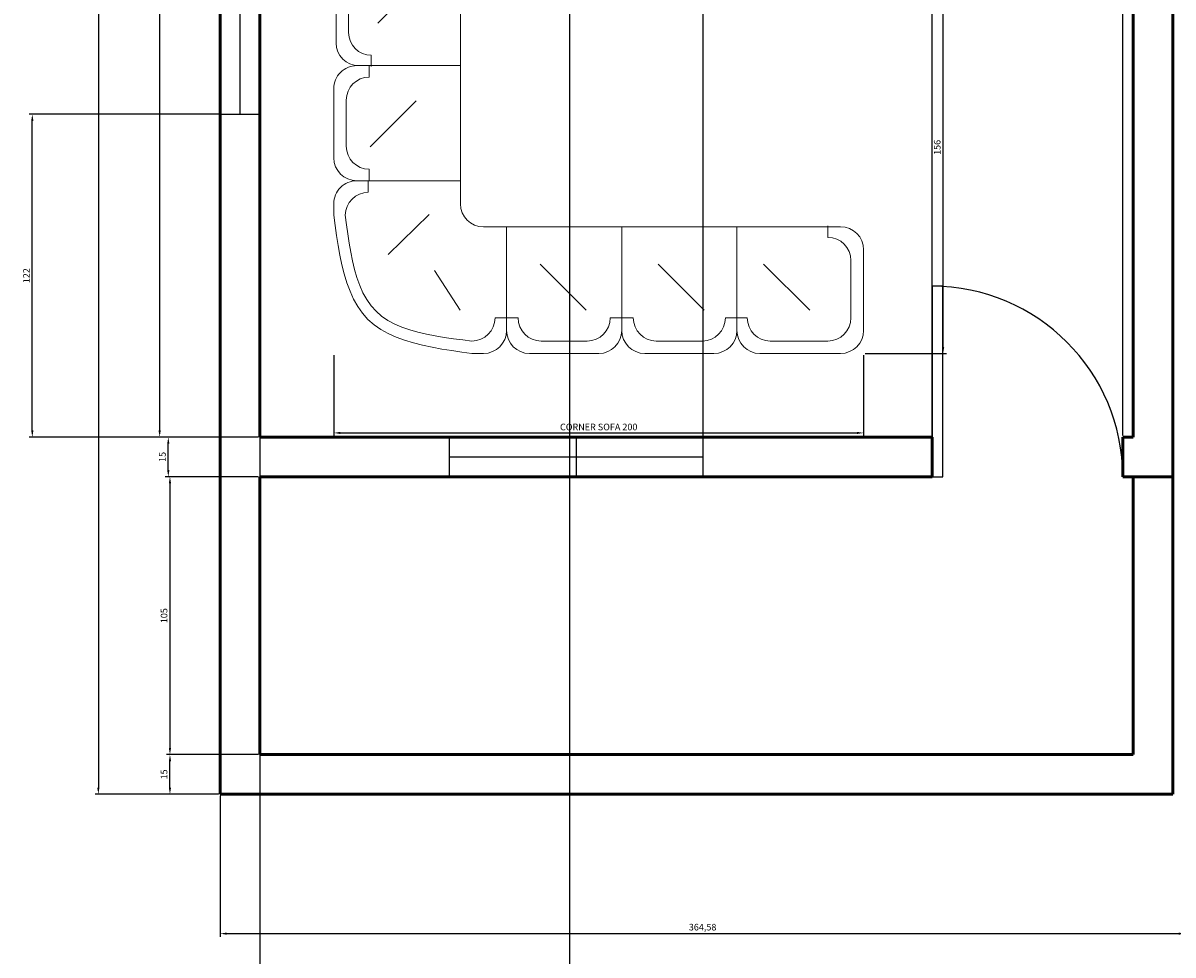
# Model space of a CAD drawing. Units: inches. Extents: x 604 to 3492, y -123 to 1737.
# Tile 2 of 20: x 604 to 1038, y 227 to 579. Entities that reach past the tile are written whole.
import ezdxf

# ---------------------------------------------------------------- set-up
doc = ezdxf.new("R2010")
doc.units = ezdxf.units.IN
for name, color, linetype, lineweight in [('A-ANNO-DIMS', 2, 'Continuous', 18), ('A-DOOR', 3, 'Continuous', 25), ('A-FURN', 8, 'Continuous', 18), ('A-GLAZ', 4, 'Continuous', 25), ('A-WALL', 7, 'Continuous', 50)]:
    doc.layers.add(name, color=color, linetype=linetype, lineweight=lineweight)
doc.styles.get("Standard").update_dxf_attribs({"font": 'arial.ttf'})
doc.dimstyles.new('ISO-25', dxfattribs={"dimtxt": 2.5, "dimasz": 2.5, "dimexe": 1.25, "dimexo": 0.625, "dimtad": 1, "dimtxsty": 'Standard', "dimcen": 2.5, "dimadec": 0, "dimazin": 0, "dimtfac": 1, "dimtmove": 0, "dimatfit": 3, "dimfxl": 1, "dimarcsym": 0})

# ---------------------------------------------------------------- blocks, each defined once
blk = doc.blocks.new('A$C4B324E0D')
for points in [[(-0.4032, -0.0374), (-0.3959, 0.0153), (-0.3883, 0.0678), (-0.3801, 0.1195), (-0.3709, 0.1704), (-0.3605, 0.22), (-0.3485, 0.2679), (-0.3346, 0.314), (-0.3185, 0.3579), (-0.2998, 0.3993), (-0.2783, 0.4378), (-0.2537, 0.4731), (-0.2255, 0.5049), (-0.1936, 0.5331), (-0.1583, 0.5578), (-0.1198, 0.5793), (-0.0785, 0.5979), (-0.0346, 0.614), (0.0115, 0.628), (0.0595, 0.64), (0.1091, 0.6504), (0.1599, 0.6595), (0.2117, 0.6678), (0.2641, 0.6753), (0.3168, 0.6826)], [(0.3768, 0.6826), (0.3168, 0.6826)], [(0.9768, 0.6826), (0.6168, 0.6826)], [(1.5769, 0.6826), (1.2168, 0.6826)], [(1.8168, 0.6826), (2.2368, 0.6826)], [(-0.3432, -0.0374), (-0.3369, 0.0114), (-0.3303, 0.0599), (-0.3232, 0.1078), (-0.3151, 0.1548), (-0.3059, 0.2006), (-0.2951, 0.2449), (-0.2826, 0.2874), (-0.2681, 0.3278), (-0.2511, 0.3658), (-0.2315, 0.4011), (-0.2089, 0.4335), (-0.1831, 0.4625), (-0.1538, 0.488), (-0.1214, 0.5102), (-0.086, 0.5294), (-0.0479, 0.546), (-0.0075, 0.5602), (0.035, 0.5722), (0.0793, 0.5825), (0.125, 0.5914), (0.172, 0.599), (0.2198, 0.6057), (0.2682, 0.6119), (0.3168, 0.6177)], [(0.3168, 0.6177), (0.3168, 0.6177)], [(0.9168, 0.6177), (0.6768, 0.6177)], [(1.5168, 0.6177), (1.2768, 0.6177)], [(2.1704, 0.6177), (1.8704, 0.6177)], [(0.4968, 0.0226), (0.4968, 0.5626)], [(0.4968, 0.5626), (0.4968, 0.0226), (1.0968, 0.0226)], [(1.0968, 0.5626), (1.0968, 0.0226), (1.6968, 0.0226)], [(1.0968, 0.0226), (1.0968, 0.5626)], [(1.6968, 0.0226), (1.6968, 0.5626)], [(2.2368, 0.0226), (1.6968, 0.0226), (1.6968, 0.5626)], [(2.3569, 0.5626), (2.3569, 0.1426)], [(0.4968, 0.4977), (0.4368, 0.4977), (0.4368, 0.4977)], [(0.5569, 0.4977), (0.5569, 0.4977), (0.4968, 0.4977)], [(1.0968, 0.4977), (1.0368, 0.4977), (1.0368, 0.4977)], [(1.1569, 0.4977), (1.1569, 0.4977), (1.0968, 0.4977)], [(1.6969, 0.4977), (1.6368, 0.4977), (1.6368, 0.4977)], [(1.7504, 0.4977), (1.7504, 0.4977), (1.6904, 0.4977)], [(2.2904, 0.1977), (2.2904, 0.4977)], [(0.255, 0.4573), (0.1211, 0.2495)], [(0.9111, 0.4573), (0.6711, 0.2173)], [(1.527, 0.4573), (1.287, 0.2173)], [(2.0759, 0.4573), (1.8359, 0.2173)], [(-0.1199, 0.1664), (0.0943, -0.0414)], [(2.1704, 0.0177), (2.1704, 0.0777), (2.1704, 0.0777)], [(0.4968, 0.0226), (0.3768, 0.0226)], [(-0.4032, -0.0974), (-0.4032, -0.0374)], [(-0.3432, -0.0374), (-0.3432, -0.0374)], [(0.2568, -0.0974), (0.2568, -0.2174)], [(-0.2232, -0.2174), (-0.2232, -0.1574), (-0.2232, -0.1574)], [(-0.2832, -0.8174), (0.2568, -0.8174), (0.2568, -0.2174)], [(0.2568, -0.2174), (-0.2832, -0.2174)], [(0.2568, -0.2174), (-0.2832, -0.2174)], [(-0.2183, -0.2174), (-0.2183, -0.2774), (-0.2183, -0.2774)], [(-0.4032, -0.3374), (-0.4032, -0.6974)], [(-0.3383, -0.3974), (-0.3383, -0.6374)], [(-0.2136, -0.3946), (0.0264, -0.6346)], [(-0.2183, -0.7574), (-0.2183, -0.7574), (-0.2183, -0.8174)], [(0.2568, -0.8174), (-0.2832, -0.8174)], [(-0.2732, -0.8174), (0.2568, -0.8174), (0.2568, -1.3475)], [(-0.208, -0.8126), (-0.208, -0.8715), (-0.208, -0.8715)], [(0.2568, -0.8174), (0.2568, -1.3475)], [(-0.391, -1.3475), (-0.391, -0.9352)], [(-0.3258, -0.9893), (-0.3258, -1.2838)], [(-0.1734, -1.0387), (0.0666, -1.2787)], [(0.2043, -1.2838), (0.2043, -1.2838), (0.2632, -1.2838)], [(-0.208, -1.4016), (0.0865, -1.4016)], [(0.1391, -1.4653), (-0.2732, -1.4653)]]:
    blk.add_lwpolyline(points)
for centre, radius, start, end in [((0.3768, 0.5626), 0.12, 0, 90), ((0.6168, 0.5626), 0.12, 90, 180), ((0.9768, 0.5626), 0.12, 0, 90), ((1.2168, 0.5626), 0.12, 90, 180), ((1.5769, 0.5626), 0.12, 0, 90), ((1.8168, 0.5626), 0.12, 90, 180), ((2.2368, 0.5626), 0.12, 0, 90), ((0.3168, 0.4977), 0.12, 0, 90), ((0.6768, 0.4977), 0.12, 90, 180), ((0.9168, 0.4977), 0.12, 0, 90), ((1.2768, 0.4977), 0.12, 90, 180), ((1.5168, 0.4977), 0.12, 0, 90), ((1.8704, 0.4977), 0.12, 90, 180), ((2.1704, 0.4977), 0.12, 0, 90), ((2.1704, 0.1977), 0.12, 270, 0), ((2.2368, 0.1426), 0.12, 270, 0), ((0.3768, -0.0974), 0.12, 90, 180), ((-0.2232, -0.0374), 0.12, 180, 270), ((-0.2832, -0.0974), 0.12, 179.9997, 270), ((-0.2832, -0.3374), 0.12, 90, 180), ((-0.2183, -0.3974), 0.12, 90, 180), ((-0.2183, -0.6374), 0.12, 180, 270), ((-0.2832, -0.6974), 0.12, 179.9997, 270), ((-0.2732, -0.9352), 0.1178, 90, 180), ((-0.208, -0.9893), 0.1178, 90, 180), ((-0.208, -1.2838), 0.1178, 180, 270), ((0.0865, -1.2838), 0.1178, 270, 0), ((-0.2732, -1.3475), 0.1178, 179.9997, 270), ((0.1391, -1.3475), 0.1178, 270, 0)]:
    blk.add_arc(centre, radius, start, end)
blk = doc.blocks.new('A$C58C6152E')
at = {"xscale": 1.5, "yscale": 1.5, "zscale": 1.5, "rotation": 90}
blk.add_blockref('A$C4B324E0D', (1.0239, 0.6047), dxfattribs=at)
blk = doc.blocks.new('A$C15DC316E')
at = {"xscale": -1, "rotation": 270}
blk.add_blockref('A$C58C6152E', (0, 0), dxfattribs=at)
blk = doc.blocks.new('*D26')
at = {"layer": 'A-ANNO-DIMS', "color": 0, "lineweight": -2, "transparency": 16777216}
for p, q in [((692.39, 762.7), (653.92, 762.7)), ((655.17, 760.2), (655.17, 425.2)), ((692.39, 422.7), (653.92, 422.7))]:
    blk.add_line(p, q, dxfattribs=at)
at = {"layer": 'A-ANNO-DIMS', "color": 0, "transparency": 16777216}
for points in [[(654.75, 760.2), (655.58, 760.2), (655.17, 762.7)], [(654.75, 425.2), (655.58, 425.2), (655.17, 422.7)]]:
    blk.add_solid(points, dxfattribs=at)
at = {"layer": 'Defpoints', "color": 0, "transparency": 16777216}
for p in [(693.01, 762.7), (655.17, 422.7), (693.01, 422.7)]:
    blk.add_point(p, dxfattribs=at)
at = {"layer": 'A-ANNO-DIMS', "color": 0, "transparency": 16777216, "insert": (653.26, 592.7), "char_height": 2.5, "attachment_point": 5, "rotation": 90}
blk.add_mtext('340', dxfattribs=at)
blk = doc.blocks.new('*D27')
at = {"layer": 'A-ANNO-DIMS', "color": 0, "lineweight": -2, "transparency": 16777216}
for p, q in [((692.39, 422.7), (657.19, 422.7)), ((658.44, 410.2), (658.44, 420.2)), ((692.39, 407.7), (657.19, 407.7))]:
    blk.add_line(p, q, dxfattribs=at)
at = {"layer": 'A-ANNO-DIMS', "color": 0, "transparency": 16777216}
for points in [[(658.02, 420.2), (658.85, 420.2), (658.44, 422.7)], [(658.02, 410.2), (658.85, 410.2), (658.44, 407.7)]]:
    blk.add_solid(points, dxfattribs=at)
at = {"layer": 'Defpoints', "color": 0, "transparency": 16777216}
for p in [(658.44, 422.7), (693.01, 422.7), (693.01, 407.7)]:
    blk.add_point(p, dxfattribs=at)
at = {"layer": 'A-ANNO-DIMS', "color": 0, "transparency": 16777216, "insert": (656.54, 415.2), "char_height": 2.5, "attachment_point": 5, "rotation": 90}
blk.add_mtext('15', dxfattribs=at)
blk = doc.blocks.new('*D28')
at = {"layer": 'A-ANNO-DIMS', "color": 0, "lineweight": -2, "transparency": 16777216}
for p, q in [((692.39, 407.7), (657.81, 407.7)), ((659.06, 405.2), (659.06, 305.2)), ((692.39, 302.7), (657.81, 302.7))]:
    blk.add_line(p, q, dxfattribs=at)
at = {"layer": 'A-ANNO-DIMS', "color": 0, "transparency": 16777216}
for points in [[(658.64, 405.2), (659.48, 405.2), (659.06, 407.7)], [(658.64, 305.2), (659.48, 305.2), (659.06, 302.7)]]:
    blk.add_solid(points, dxfattribs=at)
at = {"layer": 'Defpoints', "color": 0, "transparency": 16777216}
for p in [(693.01, 407.7), (659.06, 302.7), (693.01, 302.7)]:
    blk.add_point(p, dxfattribs=at)
at = {"layer": 'A-ANNO-DIMS', "color": 0, "transparency": 16777216, "insert": (657.16, 355.2), "char_height": 2.5, "attachment_point": 5, "rotation": 90}
blk.add_mtext('105', dxfattribs=at)
blk = doc.blocks.new('*D29')
at = {"layer": 'A-ANNO-DIMS', "color": 0, "lineweight": -2, "transparency": 16777216}
for p, q in [((677.39, 302.7), (657.81, 302.7)), ((659.06, 290.2), (659.06, 300.2)), ((677.39, 287.7), (657.81, 287.7))]:
    blk.add_line(p, q, dxfattribs=at)
at = {"layer": 'A-ANNO-DIMS', "color": 0, "transparency": 16777216}
for points in [[(658.64, 300.2), (659.48, 300.2), (659.06, 302.7)], [(658.64, 290.2), (659.48, 290.2), (659.06, 287.7)]]:
    blk.add_solid(points, dxfattribs=at)
at = {"layer": 'Defpoints', "color": 0, "transparency": 16777216}
for p in [(659.06, 302.7), (678.01, 302.7), (678.01, 287.7)]:
    blk.add_point(p, dxfattribs=at)
at = {"layer": 'A-ANNO-DIMS', "color": 0, "transparency": 16777216, "insert": (657.16, 295.2), "char_height": 2.5, "attachment_point": 5, "rotation": 90}
blk.add_mtext('15', dxfattribs=at)
blk = doc.blocks.new('*D37')
at = {"layer": 'A-ANNO-DIMS', "color": 0, "lineweight": -2, "transparency": 16777216}
for p, q in [((677.39, 1287.7), (630.76, 1287.7)), ((632.01, 1285.2), (632.01, 290.2)), ((677.39, 287.7), (630.76, 287.7))]:
    blk.add_line(p, q, dxfattribs=at)
at = {"layer": 'A-ANNO-DIMS', "color": 0, "transparency": 16777216}
for points in [[(631.59, 1285.2), (632.42, 1285.2), (632.01, 1287.7)], [(631.59, 290.2), (632.42, 290.2), (632.01, 287.7)]]:
    blk.add_solid(points, dxfattribs=at)
at = {"layer": 'Defpoints', "color": 0, "transparency": 16777216}
for p in [(678.01, 1287.7), (632.01, 287.7), (678.01, 287.7)]:
    blk.add_point(p, dxfattribs=at)
at = {"layer": 'A-ANNO-DIMS', "color": 0, "transparency": 16777216, "insert": (630.1, 787.7), "char_height": 2.5, "attachment_point": 5, "rotation": 90}
blk.add_mtext('1000', dxfattribs=at)
blk = doc.blocks.new('*D59')
at = {"layer": 'A-ANNO-DIMS', "color": 0, "lineweight": -2, "transparency": 16777216}
for p, q in [((678.01, 287.08), (678.01, 233.77)), ((1042.59, 287.08), (1042.59, 233.77)), ((680.51, 235.02), (1040.09, 235.02))]:
    blk.add_line(p, q, dxfattribs=at)
at = {"layer": 'A-ANNO-DIMS', "color": 0, "transparency": 16777216}
for points in [[(680.51, 235.44), (680.51, 234.61), (678.01, 235.02)], [(1040.09, 235.44), (1040.09, 234.61), (1042.59, 235.02)]]:
    blk.add_solid(points, dxfattribs=at)
at = {"layer": 'Defpoints', "color": 0, "transparency": 16777216}
for p in [(678.01, 287.7), (1042.59, 287.7), (1042.59, 235.02)]:
    blk.add_point(p, dxfattribs=at)
at = {"layer": 'A-ANNO-DIMS', "color": 0, "transparency": 16777216, "insert": (860.3, 237.15), "char_height": 2.5, "attachment_point": 5}
blk.add_mtext('364,58', dxfattribs=at)
blk = doc.blocks.new('DOOR-SWING-72')
for p, q in [((0, 72), (0, 0)), ((0, 0), (4, 0)), ((0, 0), (4, 0))]:
    blk.add_line(p, q)
blk.add_lwpolyline([(0, 72), (0, 0), (4, 0), (4, 72)], close=True)
blk.add_arc((0, 0), 72, 0, 90)
blk = doc.blocks.new('WIN-96')
for p, q in [((15, 96), (0, 96)), ((7.5, 96), (7.5, 0)), ((15, 96), (15, 0)), ((15, 48), (0, 48))]:
    blk.add_line(p, q)
blk.add_lwpolyline([(0, 96), (0, 0), (15, 0), (15, 96)], close=True)
blk = doc.blocks.new('*D79')
at = {"layer": 'A-ANNO-DIMS', "color": 0, "lineweight": -2, "transparency": 16777216}
for p, q in [((720.96, 453.67), (720.96, 423.02)), ((921.14, 453.67), (921.14, 423.02)), ((723.46, 424.27), (918.64, 424.27))]:
    blk.add_line(p, q, dxfattribs=at)
at = {"layer": 'A-ANNO-DIMS', "color": 0, "transparency": 16777216}
for points in [[(723.46, 424.69), (723.46, 423.86), (720.96, 424.27)], [(918.64, 424.69), (918.64, 423.86), (921.14, 424.27)]]:
    blk.add_solid(points, dxfattribs=at)
at = {"layer": 'Defpoints', "color": 0, "transparency": 16777216}
for p in [(720.96, 454.3), (921.14, 454.3), (921.14, 424.27)]:
    blk.add_point(p, dxfattribs=at)
at = {"layer": 'A-ANNO-DIMS', "color": 0, "transparency": 16777216, "insert": (821.05, 426.19), "char_height": 2.5, "attachment_point": 5}
blk.add_mtext('CORNER SOFA 200', dxfattribs=at)
blk = doc.blocks.new('*D80')
at = {"layer": 'A-ANNO-DIMS', "color": 0, "lineweight": -2, "transparency": 16777216}
for p, q in [((921.76, 610.08), (952.41, 610.08)), ((951.16, 456.8), (951.16, 607.58)), ((921.76, 454.3), (952.41, 454.3))]:
    blk.add_line(p, q, dxfattribs=at)
at = {"layer": 'A-ANNO-DIMS', "color": 0, "transparency": 16777216}
for points in [[(950.75, 607.58), (951.58, 607.58), (951.16, 610.08)], [(950.75, 456.8), (951.58, 456.8), (951.16, 454.3)]]:
    blk.add_solid(points, dxfattribs=at)
at = {"layer": 'Defpoints', "color": 0, "transparency": 16777216}
for p in [(921.14, 610.08), (951.16, 610.08), (921.14, 454.3)]:
    blk.add_point(p, dxfattribs=at)
at = {"layer": 'A-ANNO-DIMS', "color": 0, "transparency": 16777216, "insert": (949.26, 532.19), "char_height": 2.5, "attachment_point": 5, "rotation": 90}
blk.add_mtext('156', dxfattribs=at)
blk = doc.blocks.new('*D85')
at = {"layer": 'A-ANNO-DIMS', "color": 0, "lineweight": -2, "transparency": 16777216}
for p, q in [((693.01, 1272.08), (693.01, 67.77)), ((810.01, 1272.08), (810.01, 67.77)), ((695.51, 69.02), (807.51, 69.02))]:
    blk.add_line(p, q, dxfattribs=at)
at = {"layer": 'A-ANNO-DIMS', "color": 0, "transparency": 16777216}
for points in [[(695.51, 69.44), (695.51, 68.61), (693.01, 69.02)], [(807.51, 69.44), (807.51, 68.61), (810.01, 69.02)]]:
    blk.add_solid(points, dxfattribs=at)
at = {"layer": 'Defpoints', "color": 0, "transparency": 16777216}
for p in [(693.01, 1272.7), (810.01, 1272.7), (810.01, 69.02)]:
    blk.add_point(p, dxfattribs=at)
at = {"layer": 'A-ANNO-DIMS', "color": 0, "transparency": 16777216, "insert": (751.51, 70.9), "char_height": 2.5, "attachment_point": 5}
blk.add_mtext('117', dxfattribs=at)
blk = doc.blocks.new('*D89')
at = {"layer": 'A-ANNO-DIMS', "color": 0, "lineweight": -2, "transparency": 16777216}
for p, q in [((677.39, 544.7), (605.81, 544.7)), ((607.06, 425.2), (607.06, 542.2)), ((692.39, 422.7), (605.81, 422.7))]:
    blk.add_line(p, q, dxfattribs=at)
at = {"layer": 'A-ANNO-DIMS', "color": 0, "transparency": 16777216}
for points in [[(606.64, 542.2), (607.48, 542.2), (607.06, 544.7)], [(606.64, 425.2), (607.48, 425.2), (607.06, 422.7)]]:
    blk.add_solid(points, dxfattribs=at)
at = {"layer": 'Defpoints', "color": 0, "transparency": 16777216}
for p in [(607.06, 544.7), (678.01, 544.7), (693.01, 422.7)]:
    blk.add_point(p, dxfattribs=at)
at = {"layer": 'A-ANNO-DIMS', "color": 0, "transparency": 16777216, "insert": (605.18, 483.7), "char_height": 2.5, "attachment_point": 5, "rotation": 90}
blk.add_mtext('122', dxfattribs=at)
blk = doc.blocks.new('*D90')
at = {"layer": 'A-ANNO-DIMS', "color": 0, "lineweight": -2, "transparency": 16777216}
for p, q in [((1019.01, 423.33), (1019.01, 1359.9)), ((1023.01, 423.33), (1023.01, 1359.9)), ((1016.51, 1358.65), (1014.01, 1358.65)), ((1023.01, 1358.65), (1019.01, 1358.65)), ((1025.51, 1358.65), (1028.01, 1358.65))]:
    blk.add_line(p, q, dxfattribs=at)
at = {"layer": 'A-ANNO-DIMS', "color": 0, "transparency": 16777216}
for points in [[(1016.51, 1359.07), (1016.51, 1358.23), (1019.01, 1358.65)], [(1025.51, 1359.07), (1025.51, 1358.23), (1023.01, 1358.65)]]:
    blk.add_solid(points, dxfattribs=at)
at = {"layer": 'Defpoints', "color": 0, "transparency": 16777216}
for p in [(1019.01, 1358.65), (1019.01, 422.7), (1023.01, 422.7)]:
    blk.add_point(p, dxfattribs=at)
at = {"layer": 'A-ANNO-DIMS', "color": 0, "transparency": 16777216, "insert": (1021.01, 1360.53), "char_height": 2.5, "attachment_point": 5}
blk.add_mtext('4', dxfattribs=at)
blk = doc.blocks.new('*D91')
at = {"layer": 'A-ANNO-DIMS', "color": 0, "lineweight": -2, "transparency": 16777216}
for p, q in [((860.51, 408.33), (860.51, 1359.9)), ((947.01, 408.33), (947.01, 1359.9)), ((863.01, 1358.65), (944.51, 1358.65))]:
    blk.add_line(p, q, dxfattribs=at)
at = {"layer": 'A-ANNO-DIMS', "color": 0, "transparency": 16777216}
for points in [[(863.01, 1359.07), (863.01, 1358.23), (860.51, 1358.65)], [(944.51, 1359.07), (944.51, 1358.23), (947.01, 1358.65)]]:
    blk.add_solid(points, dxfattribs=at)
at = {"layer": 'Defpoints', "color": 0, "transparency": 16777216}
for p in [(947.01, 1358.65), (860.51, 407.7), (947.01, 407.7)]:
    blk.add_point(p, dxfattribs=at)
at = {"layer": 'A-ANNO-DIMS', "color": 0, "transparency": 16777216, "insert": (903.76, 1360.55), "char_height": 2.5, "attachment_point": 5}
blk.add_mtext('86.5', dxfattribs=at)

msp = doc.modelspace()

# ---------------------------------------------------------------- linework, layer by layer
at = {"layer": 'A-WALL'}
for p, q in [((678.0111, 1287.7004), (678.0111, 287.7004)), ((693.0111, 762.7004), (693.0111, 422.7004)), ((693.0111, 762.7004), (693.0111, 422.7004)), ((1038.0111, 587.7004), (1038.0111, 287.7004)), ((693.0111, 422.7004), (947.0111, 422.7004)), ((947.0111, 407.7004), (947.0111, 422.7004)), ((1019.0111, 407.7004), (1019.0111, 422.7004)), ((1019.0111, 422.7004), (1023.0111, 422.7004)), ((693.0111, 407.7004), (947.0111, 407.7004)), ((693.0111, 407.7004), (693.0111, 302.7004)), ((1019.0111, 407.7004), (1023.0111, 407.7004)), ((1023.0111, 407.7004), (1023.0111, 302.7004)), ((1023.0111, 407.7004), (1038.0111, 407.7004)), ((693.0111, 302.7004), (1023.0111, 302.7004)), ((678.0111, 287.7004), (1038.0111, 287.7004))]:
    msp.add_line(p, q, dxfattribs=at)
for points in [[(1038.0111, 602.7004), (1023.0111, 602.7004), (1023.0111, 422.7004)], [(1038.0111, 422.7004), (1038.0111, 587.7004)]]:
    msp.add_lwpolyline(points, dxfattribs=at)

# ---------------------------------------------------------------- block references
at = {"layer": 'A-DOOR'}
msp.add_blockref('DOOR-SWING-72', (947.0111, 407.7004), dxfattribs=at)
at = {"layer": 'A-FURN', "xscale": 48.35233930155243, "yscale": 48.35233930155243, "zscale": 48.35233930155243}
msp.add_blockref('A$C15DC316E', (720.9565, 454.2997), dxfattribs=at)
at = {"layer": 'A-GLAZ'}
msp.add_blockref('WIN-96', (678.0111, 544.7004), dxfattribs=at)
at = {"layer": 'A-GLAZ', "rotation": 89.99999999999991}
msp.add_blockref('WIN-96', (860.5111, 407.7004), dxfattribs=at)

# ---------------------------------------------------------------- dimensions: what is measured, and where the dimension line sits
at = {"layer": 'A-ANNO-DIMS'}
for base, p1, p2, override, picture, middle in [((947.0111, 1358.6504), (860.5111, 407.7004), (947.0111, 407.7004), {"dimdec": 1, "dimlfac": 1, "dimrnd": 0, "dimzin": 0, "dimdsep": 46, "dimlunit": 2}, '*D91', (903.7611, 1360.5519)), ((1019.0111, 1358.6504), (1023.0111, 422.7004), (1019.0111, 422.7004), {"dimdec": 0, "dimlfac": 1, "dimrnd": 0, "dimzin": 0, "dimdsep": 46, "dimlunit": 2}, '*D90', (1021.0111, 1360.5254)), ((810.0111, 69.0242), (693.0111, 1272.7004), (810.0111, 1272.7004), {"dimdec": 0, "dimlfac": 1, "dimrnd": 0, "dimzin": 0, "dimdsep": 46, "dimlunit": 2}, '*D85', (751.5111, 70.9043)), ((1042.5874, 235.0232), (678.0111, 287.7004), (1042.5874, 287.7004), {"dimclrd": 0, "dimclre": 0, "dimclrt": 0}, '*D59', (860.2993, 237.1506))]:
    dim = msp.add_linear_dim(base=base, p1=p1, p2=p2, dimstyle='ISO-25', override=override, dxfattribs=at)
    dim.commit()
    dim.dimension.update_dxf_attribs({"geometry": picture, "text_midpoint": middle})
for base, p1, p2, override, picture, middle in [((632.0054, 287.7004), (678.0111, 1287.7004), (678.0111, 287.7004), {"dimclrd": 0, "dimclre": 0, "dimclrt": 0}, '*D37', (630.104, 787.7004)), ((655.1671, 422.7004), (693.0111, 762.7004), (693.0111, 422.7004), {"dimclrd": 0, "dimclre": 0, "dimclrt": 0}, '*D26', (653.2648, 592.7004)), ((951.1628, 610.0802), (921.1359, 454.2997), (921.1359, 610.0802), {"dimdec": 0, "dimlfac": 1, "dimrnd": 0, "dimzin": 0, "dimdsep": 46, "dimlunit": 2}, '*D80', (949.2614, 532.1899)), ((607.0611, 544.7004), (693.0111, 422.7004), (678.0111, 544.7004), {"dimdec": 0, "dimlfac": 1, "dimrnd": 0, "dimzin": 0, "dimdsep": 46, "dimlunit": 2}, '*D89', (605.181, 483.7004)), ((658.4375, 422.7004), (693.0111, 407.7004), (693.0111, 422.7004), {"dimclrd": 0, "dimclre": 0, "dimclrt": 0}, '*D27', (656.5361, 415.2004)), ((659.0615, 302.7004), (693.0111, 407.7004), (693.0111, 302.7004), {"dimclrd": 0, "dimclre": 0, "dimclrt": 0}, '*D28', (657.1601, 355.2004)), ((659.0615, 302.7004), (678.0111, 287.7004), (678.0111, 302.7004), {"dimclrd": 0, "dimclre": 0, "dimclrt": 0}, '*D29', (657.1601, 295.2004))]:
    dim = msp.add_linear_dim(base=base, p1=p1, p2=p2, angle=90, dimstyle='ISO-25', override=override, dxfattribs=at)
    dim.commit()
    dim.dimension.update_dxf_attribs({"geometry": picture, "text_midpoint": middle})
dim = msp.add_linear_dim(base=(921.1359, 424.2728), p1=(720.9565, 454.2997), p2=(921.1359, 454.2997), text='CORNER SOFA <>', dimstyle='ISO-25', override={"dimdec": 0, "dimlfac": 1, "dimrnd": 0, "dimzin": 0, "dimdsep": 46, "dimlunit": 2}, dxfattribs=at)
dim.commit()
dim.dimension.update_dxf_attribs({"geometry": '*D79', "text_midpoint": (821.0462, 426.1913)})

doc.saveas('drawing.dxf')
